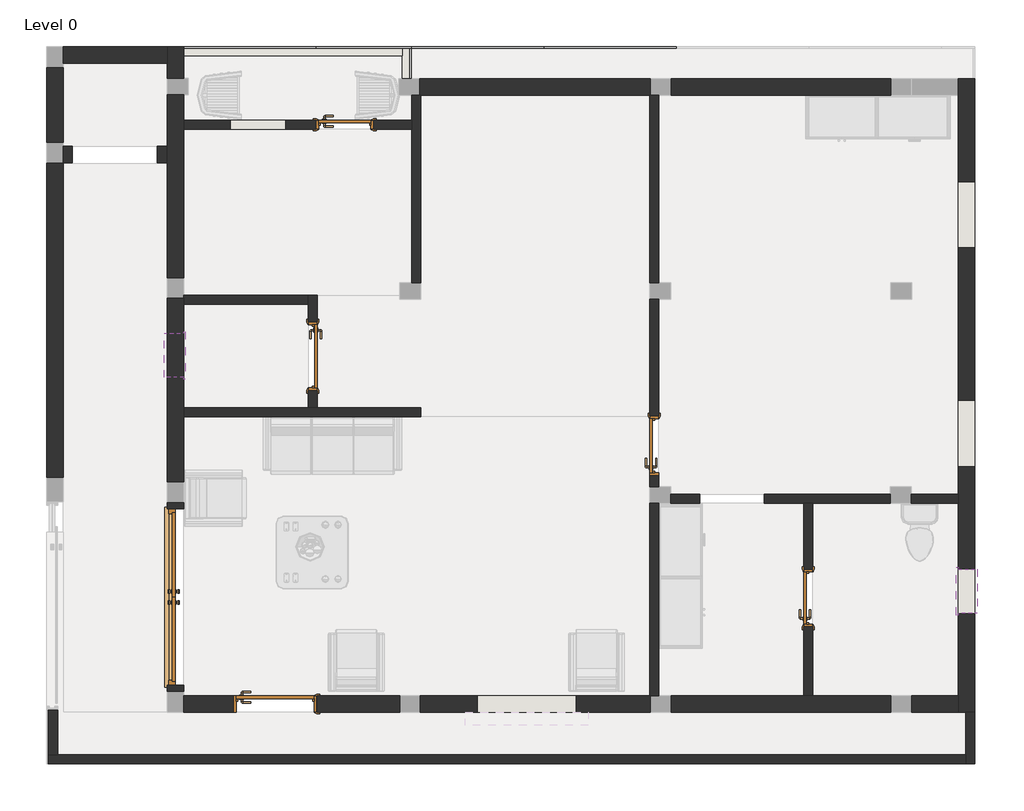
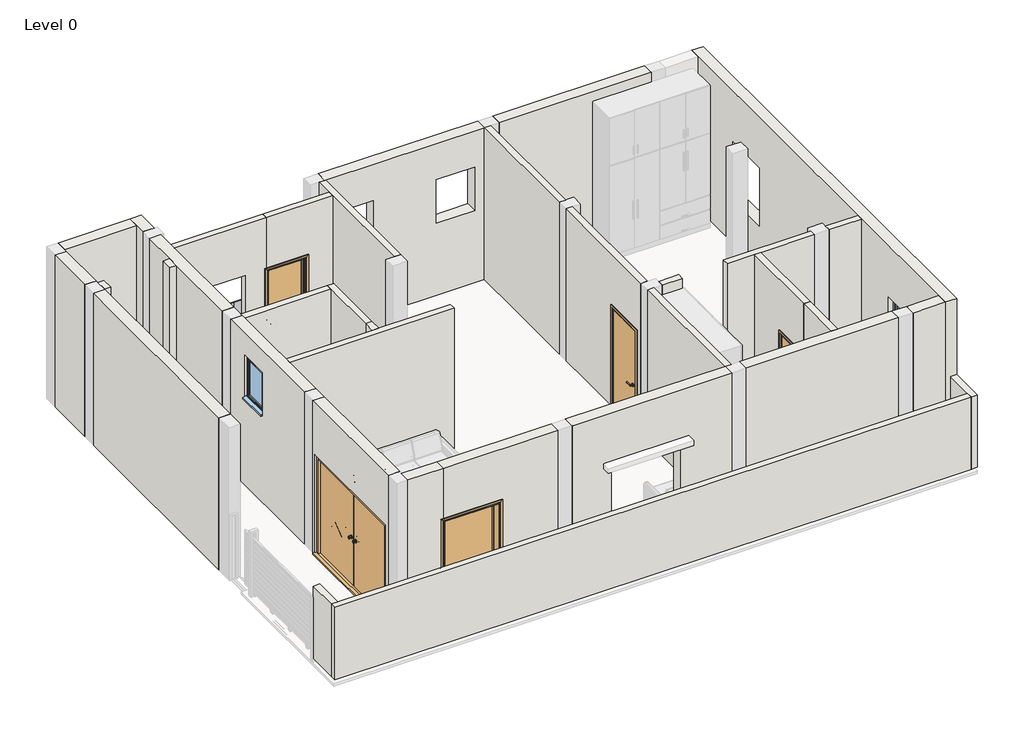
# One storey, part 1 of 2: 37 walls, 6 doors, 5 plates, 2 windows.
"""IFC4 building model written with IfcOpenShell, lengths in millimetres."""

from ifc_helpers import new_model, si_unit, frame, origin, origin_with_axes, place, context, project, spatial, polyline, outline, extrude, faceted_brep, transform, mapped, element, save
from components import doors_extdbl_flush_md_0ef74d11, doors_intsgl_d3_a25f8c6e, doors_intsgl_d4_4271d8f6, doors_intsgl_d1_afe1ebc3, doors_intsgl_d2_d6dd0e7a, system_panel_glazed_6338a664, system_panel_glazed_e6893c60, system_panel_glazed_bba74dcb, windows_sgl_plain_610x910mm_8d1346b0

model = new_model("IFC4")

# Units and contexts
model_context = context("Model", 3, world=origin())
ifc_project = project(units=[si_unit("LENGTHUNIT", "METRE", prefix="MILLI")], contexts=[model_context])

# Site, building, storey
site = spatial("IfcSite", under=ifc_project)
building = spatial("IfcBuilding", under=site)
storey = spatial("IfcBuildingStorey", under=building, Name="Level 0", Elevation=0.0)

# Doors
placement = place(None, origin())
doors_extdbl_flush_md_shape = doors_extdbl_flush_md_0ef74d11(model_context)
element("IfcDoor", 1, ObjectType="Doors_ExtDbl_Flush : MD", at=placement, inside=storey, context=model_context, shape_type="MappedRepresentation", body=[
    mapped(doors_extdbl_flush_md_shape, transform((-11061.4858712, -2060.9296054, 0.0), x_axis=(0.0, 1.0, 0.0), y_axis=(-1.0, 0.0, 0.0), z_axis=(0.0, 0.0, 1.0))),
])
doors_intsgl_d3_shape = doors_intsgl_d3_a25f8c6e(model_context)
element("IfcDoor", 2, ObjectType="Doors_IntSgl : D3", at=placement, inside=storey, context=model_context, shape_type="MappedRepresentation", body=[
    mapped(doors_intsgl_d3_shape, transform((-2315.0983223, -2074.5629976, 0.0), x_axis=(0.0, 1.0, 0.0), y_axis=(-1.0, 0.0, 0.0), z_axis=(0.0, 0.0, 1.0))),
])
element("IfcDoor", 3, ObjectType="Doors_IntSgl : D3", at=placement, inside=storey, context=model_context, shape_type="MappedRepresentation", body=[
    mapped(doors_intsgl_d3_shape, transform((-8718.3358712, 4467.3176487, 0.0), x_axis=(1.0, 0.0, 0.0), y_axis=(0.0, 1.0, 0.0), z_axis=(0.0, 0.0, 1.0))),
])
doors_intsgl_d4_shape = doors_intsgl_d4_4271d8f6(model_context)
element("IfcDoor", 4, ObjectType="Doors_IntSgl : D4", at=placement, inside=storey, context=model_context, shape_type="MappedRepresentation", body=[
    mapped(doors_intsgl_d4_shape, transform((-4442.6060272, 29.5702475, 0.0), x_axis=(0.0, 1.0, 0.0), y_axis=(-1.0, 0.0, 0.0), z_axis=(0.0, 0.0, 1.0))),
])
doors_intsgl_d1_shape = doors_intsgl_d1_afe1ebc3(model_context)
element("IfcDoor", 5, ObjectType="Doors_IntSgl : d1", at=placement, inside=storey, context=model_context, shape_type="MappedRepresentation", body=[
    mapped(doors_intsgl_d1_shape, transform((-9163.2845381, 1266.4703946, 0.0), x_axis=(0.0, -1.0, 0.0), y_axis=(1.0, 0.0, 0.0), z_axis=(0.0, 0.0, 1.0))),
])
doors_intsgl_d2_shape = doors_intsgl_d2_d6dd0e7a(model_context)
element("IfcDoor", 6, ObjectType="Doors_IntSgl : d2", at=placement, inside=storey, context=model_context, shape_type="MappedRepresentation", body=[
    mapped(doors_intsgl_d2_shape, transform((-9681.1945565, -3540.4796054, 0.0), x_axis=(1.0, 0.0, 0.0), y_axis=(0.0, 1.0, 0.0), z_axis=(0.0, 0.0, 1.0))),
])

# Plates
system_panel_glazed_shape = system_panel_glazed_6338a664(model_context)
element("IfcPlate", 7, ObjectType="System Panel : Glazed", at=placement, inside=storey, context=model_context, shape_type="MappedRepresentation", body=[
    mapped(system_panel_glazed_shape, transform((-10032.185871, 5496.5824405, 0.0), x_axis=(1.0, 0.0, 0.0), y_axis=(0.0, 1.0, 0.0), z_axis=(0.0, 0.0, 1.0))),
])
element("IfcPlate", 8, ObjectType="System Panel : Glazed", at=placement, inside=storey, context=model_context, shape_type="MappedRepresentation", body=[
    mapped(system_panel_glazed_shape, transform((-6883.885871, 5497.0125322, 0.0), x_axis=(1.0, 0.0, 0.0), y_axis=(0.0, 1.0, 0.0), z_axis=(0.0, 0.0, 1.0))),
])
element("IfcPlate", 9, ObjectType="System Panel : Glazed", at=placement, inside=storey, context=model_context, shape_type="MappedRepresentation", body=[
    mapped(system_panel_glazed_shape, transform((-5053.8858709, 5497.0125322, 0.0), x_axis=(1.0, 0.0, 0.0), y_axis=(0.0, 1.0, 0.0), z_axis=(0.0, 0.0, 1.0))),
])
system_panel_glazed_2_shape = system_panel_glazed_e6893c60(model_context)
element("IfcPlate", 10, ObjectType="System Panel : Glazed", at=placement, inside=storey, context=model_context, shape_type="MappedRepresentation", body=[
    mapped(system_panel_glazed_2_shape, transform((-8458.035871, 5496.5824405, 0.0), x_axis=(1.0, 0.0, 0.0), y_axis=(0.0, 1.0, 0.0), z_axis=(0.0, 0.0, 1.0))),
])
system_panel_glazed_3_shape = system_panel_glazed_bba74dcb(model_context)
element("IfcPlate", 11, ObjectType="System Panel : Glazed", at=placement, inside=storey, context=model_context, shape_type="MappedRepresentation", body=[
    mapped(system_panel_glazed_3_shape, transform((-7848.3858712, 5311.357594, 0.0), x_axis=(0.0, -1.0, 0.0), y_axis=(1.0, 0.0, 0.0), z_axis=(0.0, 0.0, 1.0))),
])

# Walls
element("IfcWall", 12, ObjectType="5\"", at=placement, inside=storey, context=model_context, shape_type="SweptSolid", body=[
    extrude(outline(polyline([(-10947.1858712, 5546.4824405), (-7926.5134981, 5546.4824405), (-7926.5134981, 5419.4824405), (-10947.1858712, 5419.4824405), (-10947.1858712, 5546.4824405)])), origin_with_axes(), (0.0, 0.0, 1.0), 76.2),
])
element("IfcWall", 13, ObjectType="5\"", at=placement, inside=storey, context=model_context, shape_type="SweptSolid", body=[
    extrude(outline(polyline([(-7926.5134981, 5101.6327475), (-7926.5134981, 5546.4824405), (-7799.5134981, 5546.4824405), (-7799.5134981, 5101.6327475), (-7926.5134981, 5101.6327475)])), origin_with_axes(), (0.0, 0.0, 1.0), 76.2),
])
element("IfcWall", 14, ObjectType="5\"", at=placement, inside=storey, context=model_context, shape_type="Brep", body=[
    faceted_brep([(-140.83523, -3654.7796054, 76.2), (-140.83523, -4238.9796054, 76.2), (-140.83523, -4365.9796054, 76.2), (-140.83523, -4365.9796054, 1600.2), (-140.83523, -4238.9796054, 1600.2), (-140.83523, -3654.7796054, 1600.2), (-13.83523, -3654.7796054, 76.2), (-13.83523, -3654.7796054, 1600.2), (-13.83523, -4365.9796054, 1600.2), (-13.83523, -4365.9796054, 76.2)], [[[0, 1, 2, 3, 4, 5]], [[6, 7, 8, 9]], [[2, 1, 0, 6, 9]], [[3, 2, 9, 8]], [[5, 4, 3, 8, 7]], [[0, 5, 7, 6]]]),
])
element("IfcWall", 15, ObjectType="5\"", at=placement, inside=storey, context=model_context, shape_type="Brep", body=[
    faceted_brep([(-140.83523, -4238.9796054, 76.2), (-12688.43523, -4238.9796054, 76.2), (-12815.43523, -4238.9796054, 76.2), (-12815.43523, -4238.9796054, 1600.2), (-12688.43523, -4238.9796054, 1600.2), (-140.83523, -4238.9796054, 1600.2), (-140.83523, -4365.9796054, 76.2), (-140.83523, -4365.9796054, 1600.2), (-12815.43523, -4365.9796054, 1600.2), (-12815.43523, -4365.9796054, 76.2)], [[[0, 1, 2, 3, 4, 5]], [[6, 7, 8, 9]], [[2, 1, 0, 6, 9]], [[3, 2, 9, 8]], [[5, 4, 3, 8, 7]], [[0, 5, 7, 6]]]),
])
element("IfcWall", 16, ObjectType="5\"", at=placement, inside=storey, context=model_context, shape_type="SweptSolid", body=[
    extrude(outline(polyline([(-12688.43523, -3623.9896501), (-12688.43523, -4238.9796054), (-12815.43523, -4238.9796054), (-12815.43523, -3623.9896501), (-12688.43523, -3623.9896501)])), frame((0.0, 0.0, 76.2), z_axis=(0.0, 0.0, 1.0), x_axis=(1.0, 0.0, 0.0)), (0.0, 0.0, 1.0), 1524.0),
])
element("IfcWall", 17, ObjectType="9\"", at=placement, inside=storey, context=model_context, shape_type="SweptSolid", body=[
    extrude(outline(polyline([(-12836.0604224, 4222.4988089), (-12836.0604224, 5253.6949405), (-12607.4604224, 5253.6949405), (-12607.4604224, 4222.4988089), (-12836.0604224, 4222.4988089)])), origin_with_axes(), (0.0, 0.0, 1.0), 3200.4),
])
element("IfcWall", 18, ObjectType="9\"", at=placement, inside=storey, context=model_context, shape_type="SweptSolid", body=[
    extrude(outline(polyline([(-12836.0604224, -404.5396501), (-12836.0604224, 3930.3988089), (-12607.4604224, 3930.3988089), (-12607.4604224, -404.5396501), (-12836.0604224, -404.5396501)])), origin_with_axes(), (0.0, 0.0, 1.0), 3200.4),
])
element("IfcWall", 19, ObjectType="9\"", at=placement, inside=storey, context=model_context, shape_type="SweptSolid", body=[
    extrude(outline(polyline([(3200.4, -10240.7910021), (3200.4, -10947.1858712), (0.0, -10947.1858712), (0.0, -10259.0445565), (2110.0, -10259.0445565), (2110.0, -10240.7910021), (3200.4, -10240.7910021)])), frame((0.0, -3654.7796054, 0.0), z_axis=(0.0, 1.0, 0.0), x_axis=(0.0, 0.0, 1.0)), (0.0, 0.0, 1.0), 228.6),
])
element("IfcWall", 20, ObjectType="9\"", at=placement, inside=storey, context=model_context, shape_type="SweptSolid", body=[
    extrude(outline(polyline([(0.0, -7960.3445565), (3200.4, -7960.3445565), (3200.4, -10240.7910021), (2110.0, -10240.7910021), (2110.0, -9103.3445565), (0.0, -9103.3445565), (0.0, -7960.3445565)])), frame((0.0, -3654.7796054, 0.0), z_axis=(0.0, 1.0, 0.0), x_axis=(0.0, 0.0, 1.0)), (0.0, 0.0, 1.0), 228.6),
])
element("IfcWall", 21, ObjectType="9\"", at=placement, inside=storey, context=model_context, shape_type="SweptSolid", body=[
    extrude(outline(polyline([(0.0, -7678.28523), (0.0, -4496.93523), (3200.4, -4496.93523), (3200.4, -7678.28523), (0.0, -7678.28523)]), holes=[polyline([(2133.6, -6890.88523), (2133.6, -5519.28523), (914.4, -5519.28523), (914.4, -6890.88523), (2133.6, -6890.88523)])]), frame((0.0, -3654.7796054, 0.0), z_axis=(0.0, 1.0, 0.0), x_axis=(0.0, 0.0, 1.0)), (0.0, 0.0, 1.0), 228.6),
])
element("IfcWall", 22, ObjectType="9\"", at=placement, inside=storey, context=model_context, shape_type="SweptSolid", body=[
    extrude(outline(polyline([(-1175.88523, -3654.7796054), (-4204.83523, -3654.7796054), (-4204.83523, -3426.1796054), (-1175.88523, -3426.1796054), (-1175.88523, -3654.7796054)])), origin_with_axes(), (0.0, 0.0, 1.0), 3200.4),
])
element("IfcWall", 23, ObjectType="9\"", at=placement, inside=storey, context=model_context, shape_type="SweptSolid", body=[
    extrude(outline(polyline([(-242.43523, -3654.7796054), (-883.78523, -3654.7796054), (-883.78523, -3426.1796054), (-242.43523, -3426.1796054), (-242.43523, -3654.7796054)])), origin_with_axes(), (0.0, 0.0, 1.0), 3200.4),
])
element("IfcWall", 24, ObjectType="9\"", at=placement, inside=storey, context=model_context, shape_type="Brep", body=[
    faceted_brep([(-13.83523, -3654.7796054, 0.0), (-13.83523, 5101.6327475, 0.0), (-13.83523, 5101.6327475, 3200.4), (-13.83523, -3654.7796054, 3200.4), (-13.83523, -3654.7796054, 1600.2), (-13.83523, -3654.7796054, 76.2), (-13.83523, 2764.8327475, 2133.6), (-13.83523, 3679.2327475, 2133.6), (-13.83523, 3679.2327475, 914.4), (-13.83523, 2764.8327475, 914.4), (-13.83523, -257.7672525, 2133.6), (-13.83523, 656.6327475, 2133.6), (-13.83523, 656.6327475, 914.4), (-13.83523, -257.7672525, 914.4), (-13.83523, -1676.8734289, 2110.0), (-13.83523, -1676.8734289, 1200.0), (-13.83523, -2286.4734289, 1200.0), (-13.83523, -2286.4734289, 2110.0), (-242.43523, -3654.7796054, 0.0), (-242.43523, -3654.7796054, 3200.4), (-242.43523, -3426.1796054, 3200.4), (-242.43523, 4873.0327475, 3200.4), (-242.43523, 5101.6327475, 3200.4), (-242.43523, 5101.6327475, 0.0), (-242.43523, 4873.0327475, 0.0), (-242.43523, -3426.1796054, 0.0), (-242.43523, 2764.8327475, 2133.6), (-242.43523, 2764.8327475, 914.4), (-242.43523, 3679.2327475, 914.4), (-242.43523, 3679.2327475, 2133.6), (-242.43523, -257.7672525, 2133.6), (-242.43523, -257.7672525, 914.4), (-242.43523, 656.6327475, 914.4), (-242.43523, 656.6327475, 2133.6), (-242.43523, -1676.8734289, 2110.0), (-242.43523, -2286.4734289, 2110.0), (-242.43523, -2286.4734289, 1200.0), (-242.43523, -1676.8734289, 1200.0)], [[[0, 1, 2, 3, 4, 5], [6, 7, 8, 9], [10, 11, 12, 13], [14, 15, 16, 17]], [[18, 19, 20, 21, 22, 23, 24, 25], [26, 27, 28, 29], [30, 31, 32, 33], [34, 35, 36, 37]], [[1, 0, 18, 25, 24, 23]], [[2, 1, 23, 22]], [[3, 2, 22, 21, 20, 19]], [[0, 5, 4, 3, 19, 18]], [[27, 26, 6, 9]], [[28, 27, 9, 8]], [[29, 28, 8, 7]], [[26, 29, 7, 6]], [[31, 30, 10, 13]], [[32, 31, 13, 12]], [[33, 32, 12, 11]], [[30, 33, 11, 10]], [[15, 14, 34, 37]], [[16, 15, 37, 36]], [[17, 16, 36, 35]], [[14, 17, 35, 34]]]),
])
element("IfcWall", 25, ObjectType="9\"", at=placement, inside=storey, context=model_context, shape_type="SweptSolid", body=[
    extrude(outline(polyline([(-4207.375513, 5101.6327475), (-1175.88523, 5101.6327475), (-1175.88523, 4873.0327475), (-4207.375513, 4873.0327475), (-4207.375513, 5101.6327475)])), origin_with_axes(), (0.0, 0.0, 1.0), 3200.4),
])
element("IfcWall", 26, ObjectType="9\"", at=placement, inside=storey, context=model_context, shape_type="Brep", body=[
    faceted_brep([(-4499.475513, 5101.6327475, 0.0), (-7680.825513, 5101.6327475, 0.0), (-7680.825513, 5101.6327475, 3200.4), (-4499.475513, 5101.6327475, 3200.4), (-7477.625513, 5101.6327475, 2438.4), (-7477.625513, 5101.6327475, 1524.0), (-6715.625513, 5101.6327475, 1524.0), (-6715.625513, 5101.6327475, 2438.4), (-5458.325513, 5101.6327475, 2438.4), (-5458.325513, 5101.6327475, 1524.0), (-4696.325513, 5101.6327475, 1524.0), (-4696.325513, 5101.6327475, 2438.4), (-4499.475513, 4873.0327475, 0.0), (-4499.475513, 4873.0327475, 3200.4), (-7666.1634981, 4873.0327475, 3200.4), (-7680.825513, 4873.0327475, 3200.4), (-7680.825513, 4873.0327475, 0.0), (-7666.1634981, 4873.0327475, 0.0), (-7477.625513, 4873.0327475, 2438.4), (-6715.625513, 4873.0327475, 2438.4), (-6715.625513, 4873.0327475, 1524.0), (-7477.625513, 4873.0327475, 1524.0), (-5458.325513, 4873.0327475, 2438.4), (-4696.325513, 4873.0327475, 2438.4), (-4696.325513, 4873.0327475, 1524.0), (-5458.325513, 4873.0327475, 1524.0)], [[[0, 1, 2, 3], [4, 5, 6, 7], [8, 9, 10, 11]], [[12, 13, 14, 15, 16, 17], [18, 19, 20, 21], [22, 23, 24, 25]], [[1, 0, 12, 17, 16]], [[2, 1, 16, 15]], [[3, 2, 15, 14, 13]], [[0, 3, 13, 12]], [[5, 4, 18, 21]], [[6, 5, 21, 20]], [[7, 6, 20, 19]], [[4, 7, 19, 18]], [[9, 8, 22, 25]], [[10, 9, 25, 24]], [[11, 10, 24, 23]], [[8, 11, 23, 22]]]),
])
element("IfcWall", 27, ObjectType="9\"", at=placement, inside=storey, context=model_context, shape_type="SweptSolid", body=[
    extrude(outline(polyline([(-11175.7858712, 5317.1949405), (-12607.4604224, 5317.1949405), (-12607.4604224, 5545.7949405), (-11175.7858712, 5545.7949405), (-11175.7858712, 5317.1949405)])), origin_with_axes(), (0.0, 0.0, 1.0), 3200.4),
])
element("IfcWall", 28, ObjectType="9\"", at=placement, inside=storey, context=model_context, shape_type="Brep", body=[
    faceted_brep([(-11175.7858712, 5545.7949405, 0.0), (-11175.7858712, 5317.1949405, 0.0), (-11175.7858712, 5105.4926487, 0.0), (-11175.7858712, 5105.4926487, 3200.4), (-11175.7858712, 5317.1949405, 3200.4), (-11175.7858712, 5545.7949405, 3200.4), (-10947.1858712, 5545.7949405, 0.0), (-10947.1858712, 5545.7949405, 3200.4), (-10947.1858712, 5105.4926487, 3200.4), (-10947.1858712, 5105.4926487, 0.0)], [[[0, 1, 2, 3, 4, 5]], [[6, 7, 8, 9]], [[2, 1, 0, 6, 9]], [[3, 2, 9, 8]], [[5, 4, 3, 8, 7]], [[0, 5, 7, 6]]]),
])
element("IfcWall", 29, ObjectType="9\"", at=placement, inside=storey, context=model_context, shape_type="Brep", body=[
    faceted_brep([(-11175.7858712, 4876.8926487, 0.0), (-11175.7858712, 4168.5238089, 0.0), (-11175.7858712, 3939.9238089, 0.0), (-11175.7858712, 2353.0673305, 0.0), (-11175.7858712, 2353.0673305, 3200.4), (-11175.7858712, 3939.9238089, 3200.4), (-11175.7858712, 4168.5238089, 3200.4), (-11175.7858712, 4876.8926487, 3200.4), (-10947.1858712, 4876.8926487, 0.0), (-10947.1858712, 4876.8926487, 3200.4), (-10947.1858712, 4530.8176487, 3200.4), (-10947.1858712, 4403.8176487, 3200.4), (-10947.1858712, 2353.0673305, 3200.4), (-10947.1858712, 2353.0673305, 0.0), (-10947.1858712, 4403.8176487, 0.0), (-10947.1858712, 4530.8176487, 0.0)], [[[0, 1, 2, 3, 4, 5, 6, 7]], [[8, 9, 10, 11, 12, 13, 14, 15]], [[3, 2, 1, 0, 8, 15, 14, 13]], [[4, 3, 13, 12]], [[7, 6, 5, 4, 12, 11, 10, 9]], [[0, 7, 9, 8]]]),
])
element("IfcWall", 30, ObjectType="9\"", at=placement, inside=storey, context=model_context, shape_type="SweptSolid", body=[
    extrude(outline(polyline([(2065.5455124, 0.0), (-467.0796054, 0.0), (-467.0796054, 3200.4), (2065.5455124, 3200.4), (2065.5455124, 0.0)]), holes=[polyline([(973.3455124, 2738.8), (973.3455124, 1828.8), (1582.9455124, 1828.8), (1582.9455124, 2738.8), (973.3455124, 2738.8)])]), frame((-11175.7858712, 0.0, 0.0), z_axis=(1.0, 0.0, 0.0), x_axis=(0.0, 1.0, 0.0)), (0.0, 0.0, 1.0), 228.6),
])
element("IfcWall", 31, ObjectType="9\"", at=placement, inside=storey, context=model_context, shape_type="SweptSolid", body=[
    extrude(outline(polyline([(-759.1796054, 0.0), (-841.7296054, 0.0), (-841.7296054, 2110.0), (-3280.1296054, 2110.0), (-3280.1296054, 0.0), (-3362.6796054, 0.0), (-3362.6796054, 3200.4), (-759.1796054, 3200.4), (-759.1796054, 0.0)])), frame((-11175.7858712, 0.0, 0.0), z_axis=(1.0, 0.0, 0.0), x_axis=(0.0, 1.0, 0.0)), (0.0, 0.0, 1.0), 228.6),
])
element("IfcWall", 32, ObjectType="9\"", at=placement, inside=storey, context=model_context, shape_type="SweptSolid", body=[
    extrude(outline(polyline([(-12486.8104224, 3939.9238089), (-12607.4604224, 3939.9238089), (-12607.4604224, 4168.5238089), (-12486.8104224, 4168.5238089), (-12486.8104224, 3939.9238089)])), origin_with_axes(), (0.0, 0.0, 1.0), 3200.4),
])
element("IfcWall", 33, ObjectType="9\"", at=placement, inside=storey, context=model_context, shape_type="SweptSolid", body=[
    extrude(outline(polyline([(-11175.7858712, 3939.9238089), (-11308.4687707, 3939.9238089), (-11308.4687707, 4168.5238089), (-11175.7858712, 4168.5238089), (-11175.7858712, 3939.9238089)])), origin_with_axes(), (0.0, 0.0, 1.0), 3200.4),
])
element("IfcWall", 34, ObjectType="brick 5\"", at=placement, inside=storey, context=model_context, shape_type="SweptSolid", body=[
    extrude(outline(polyline([(0.0, -10947.1858712), (0.0, -9118.3858712), (3200.4, -9118.3858712), (3200.4, -10947.1858712), (0.0, -10947.1858712)]), holes=[polyline([(2133.6, -10299.4858712), (2133.6, -9537.4858712), (914.4, -9537.4858712), (914.4, -10299.4858712), (2133.6, -10299.4858712)])]), frame((0.0, 4403.8176487, 0.0), z_axis=(0.0, 1.0, 0.0), x_axis=(0.0, 0.0, 1.0)), (0.0, 0.0, 1.0), 127.0),
])
element("IfcWall", 35, ObjectType="brick 5\"", at=placement, inside=storey, context=model_context, shape_type="SweptSolid", body=[
    extrude(outline(polyline([(0.0, -7793.1634981), (3200.4, -7793.1634981), (3200.4, -9118.3858712), (2110.0, -9118.3858712), (2110.0, -8318.2858712), (0.0, -8318.2858712), (0.0, -7793.1634981)])), frame((0.0, 4403.8176487, 0.0), z_axis=(0.0, 1.0, 0.0), x_axis=(0.0, 0.0, 1.0)), (0.0, 0.0, 1.0), 127.0),
])
element("IfcWall", 36, ObjectType="brick 5\"", at=placement, inside=storey, context=model_context, shape_type="Brep", body=[
    faceted_brep([(-7793.1634981, 4873.0327475, 0.0), (-7793.1634981, 4530.8176487, 0.0), (-7793.1634981, 4403.8176487, 0.0), (-7793.1634981, 2285.4077475, 0.0), (-7793.1634981, 2285.4077475, 3200.4), (-7793.1634981, 4403.8176487, 3200.4), (-7793.1634981, 4530.8176487, 3200.4), (-7793.1634981, 4873.0327475, 3200.4), (-7666.1634981, 4873.0327475, 0.0), (-7666.1634981, 4873.0327475, 3200.4), (-7666.1634981, 2285.4077475, 3200.4), (-7666.1634981, 2285.4077475, 0.0), (-7680.825513, 4873.0327475, 0.0), (-7680.825513, 4873.0327475, 3200.4)], [[[0, 1, 2, 3, 4, 5, 6, 7]], [[8, 9, 10, 11]], [[3, 2, 1, 0, 12, 8, 11]], [[4, 3, 11, 10]], [[7, 6, 5, 4, 10, 9, 13]], [[0, 7, 13, 9, 8, 12]]]),
])
element("IfcWall", 37, ObjectType="brick 5\"", at=placement, inside=storey, context=model_context, shape_type="SweptSolid", body=[
    extrude(outline(polyline([(-9226.7845381, 1983.7280605), (-10947.1858712, 1983.7280605), (-10947.1858712, 2110.7280605), (-9226.7845381, 2110.7280605), (-9226.7845381, 1983.7280605)])), origin_with_axes(), (0.0, 0.0, 1.0), 3200.4),
])
element("IfcWall", 38, ObjectType="brick 5\"", at=placement, inside=storey, context=model_context, shape_type="Brep", body=[
    faceted_brep([(-9226.7845381, 790.2203946, 3200.4), (-9226.7845381, 1983.7280605, 3200.4), (-9226.7845381, 2110.7280605, 3200.4), (-9226.7845381, 2110.7280605, 0.0), (-9226.7845381, 1983.7280605, 0.0), (-9226.7845381, 1742.7203946, 0.0), (-9226.7845381, 1742.7203946, 2110.0), (-9226.7845381, 790.2203946, 2110.0), (-9099.7845381, 2110.7280605, 3200.4), (-9099.7845381, 790.2203946, 3200.4), (-9099.7845381, 790.2203946, 2110.0), (-9099.7845381, 1742.7203946, 2110.0), (-9099.7845381, 1742.7203946, 0.0), (-9099.7845381, 2110.7280605, 0.0)], [[[0, 1, 2, 3, 4, 5, 6, 7]], [[8, 9, 10, 11, 12, 13]], [[3, 13, 12, 5, 4]], [[9, 0, 7, 10]], [[2, 1, 0, 9, 8]], [[3, 2, 8, 13]], [[6, 11, 10, 7]], [[11, 6, 5, 12]]]),
])
element("IfcWall", 39, ObjectType="brick 5\"", at=placement, inside=storey, context=model_context, shape_type="Brep", body=[
    faceted_brep([(-10947.1858712, 428.2703946, 0.0), (-7670.5858712, 428.2703946, 0.0), (-7670.5858712, 428.2703946, 3200.4), (-10947.1858712, 428.2703946, 3200.4), (-10947.1858712, 555.2703946, 0.0), (-10947.1858712, 555.2703946, 3200.4), (-9226.3358712, 555.2703946, 3200.4), (-9099.3358712, 555.2703946, 3200.4), (-7670.5858712, 555.2703946, 3200.4), (-7670.5858712, 555.2703946, 0.0), (-9099.3358712, 555.2703946, 0.0), (-9226.3358712, 555.2703946, 0.0)], [[[0, 1, 2, 3]], [[4, 5, 6, 7, 8, 9, 10, 11]], [[1, 0, 4, 11, 10, 9]], [[2, 1, 9, 8]], [[3, 2, 8, 7, 6, 5]], [[0, 3, 5, 4]]]),
])
element("IfcWall", 40, ObjectType="brick 5\"", at=placement, inside=storey, context=model_context, shape_type="SweptSolid", body=[
    extrude(outline(polyline([(-9099.3358712, 790.2203946), (-9099.3358712, 555.2703946), (-9226.3358712, 555.2703946), (-9226.3358712, 790.2203946), (-9099.3358712, 790.2203946)])), origin_with_axes(), (0.0, 0.0, 1.0), 3200.4),
])
element("IfcWall", 41, ObjectType="brick 5\"", at=placement, inside=storey, context=model_context, shape_type="SweptSolid", body=[
    extrude(outline(polyline([(-4506.1060272, 2285.4077475), (-4506.1060272, 4873.0327475), (-4379.1060272, 4873.0327475), (-4379.1060272, 2285.4077475), (-4506.1060272, 2285.4077475)])), origin_with_axes(), (0.0, 0.0, 1.0), 3200.4),
])
element("IfcWall", 42, ObjectType="brick 5\"", at=placement, inside=storey, context=model_context, shape_type="SweptSolid", body=[
    extrude(outline(polyline([(-535.5797525, 0.0), (-535.5797525, 3200.4), (2056.8077475, 3200.4), (2056.8077475, 0.0), (442.3202475, 0.0), (442.3202475, 2110.0), (-383.1797525, 2110.0), (-383.1797525, 0.0), (-535.5797525, 0.0)])), frame((-4506.1060272, 0.0, 0.0), z_axis=(1.0, 0.0, 0.0), x_axis=(0.0, 1.0, 0.0)), (0.0, 0.0, 1.0), 127.0),
])
element("IfcWall", 43, ObjectType="brick 5\"", at=placement, inside=storey, context=model_context, shape_type="SweptSolid", body=[
    extrude(outline(polyline([(-4506.1060272, -3426.1796054), (-4506.1060272, -764.1797525), (-4379.1060272, -764.1797525), (-4379.1060272, -3426.1796054), (-4506.1060272, -3426.1796054)])), origin_with_axes(), (0.0, 0.0, 1.0), 3200.4),
])
element("IfcWall", 44, ObjectType="brick 5\"", at=placement, inside=storey, context=model_context, shape_type="SweptSolid", body=[
    extrude(outline(polyline([(-3813.9560272, -764.1797525), (-4214.0060272, -764.1797525), (-4214.0060272, -637.1797525), (-3813.9560272, -637.1797525), (-3813.9560272, -764.1797525)])), origin_with_axes(), (0.0, 0.0, 1.0), 3200.4),
])
element("IfcWall", 45, ObjectType="brick 5\"", at=placement, inside=storey, context=model_context, shape_type="Brep", body=[
    faceted_brep([(-2920.6153893, -764.1797525, 0.0), (-2378.5983223, -764.1797525, 0.0), (-2251.5983223, -764.1797525, 0.0), (-1182.23523, -764.1797525, 0.0), (-1182.23523, -764.1797525, 3200.4), (-2251.5983223, -764.1797525, 3200.4), (-2378.5983223, -764.1797525, 3200.4), (-2920.6153893, -764.1797525, 3200.4), (-2920.6153893, -637.1797525, 0.0), (-2920.6153893, -637.1797525, 3200.4), (-1182.23523, -637.1797525, 3200.4), (-1182.23523, -637.1797525, 0.0)], [[[0, 1, 2, 3, 4, 5, 6, 7]], [[8, 9, 10, 11]], [[3, 2, 1, 0, 8, 11]], [[4, 3, 11, 10]], [[7, 6, 5, 4, 10, 9]], [[0, 7, 9, 8]]]),
])
element("IfcWall", 46, ObjectType="brick 5\"", at=placement, inside=storey, context=model_context, shape_type="SweptSolid", body=[
    extrude(outline(polyline([(-242.43523, -764.1797525), (-890.13523, -764.1797525), (-890.13523, -637.1797525), (-242.43523, -637.1797525), (-242.43523, -764.1797525)])), origin_with_axes(), (0.0, 0.0, 1.0), 3200.4),
])
element("IfcWall", 47, ObjectType="brick 5\"", at=placement, inside=storey, context=model_context, shape_type="SweptSolid", body=[
    extrude(outline(polyline([(-2474.6129976, 3200.4), (-764.1797525, 3200.4), (-764.1797525, 0.0), (-1674.5129976, 0.0), (-1674.5129976, 2110.0), (-2474.6129976, 2110.0), (-2474.6129976, 3200.4)])), frame((-2378.5983223, 0.0, 0.0), z_axis=(1.0, 0.0, 0.0), x_axis=(0.0, 1.0, 0.0)), (0.0, 0.0, 1.0), 127.0),
])
element("IfcWall", 48, ObjectType="brick 5\"", at=placement, inside=storey, context=model_context, shape_type="SweptSolid", body=[
    extrude(outline(polyline([(-2378.5983223, -3426.1796054), (-2378.5983223, -2474.6129976), (-2251.5983223, -2474.6129976), (-2251.5983223, -3426.1796054), (-2378.5983223, -3426.1796054)])), origin_with_axes(), (0.0, 0.0, 1.0), 3200.4),
])

# Windows
windows_sgl_plain_610x910mm_shape = windows_sgl_plain_610x910mm_8d1346b0(model_context)
element("IfcWindow", 49, ObjectType="Windows_Sgl_Plain : 610x910mm", at=placement, inside=storey, context=model_context, shape_type="MappedRepresentation", body=[
    mapped(windows_sgl_plain_610x910mm_shape, transform((-11053.0293033, 1278.1455124, 628.8), x_axis=(0.0, 1.0, 0.0), y_axis=(-1.0, 0.0, 0.0), z_axis=(0.0, 0.0, 1.0))),
])
element("IfcWindow", 50, ObjectType="Windows_Sgl_Plain : 610x910mm", at=placement, inside=storey, context=model_context, shape_type="MappedRepresentation", body=[
    mapped(windows_sgl_plain_610x910mm_shape, transform((-136.5917978, -1981.6734289, 0.0), x_axis=(0.0, -1.0, 0.0), y_axis=(1.0, 0.0, 0.0), z_axis=(0.0, 0.0, 1.0))),
])

save(model, "model.ifc")

# Revit data of these elements
# Type "Doors_ExtDbl_Flush : MD"
#   Type Mark = "47"
#   Type Comments = "External Double"
#   Operation = "DoubleDoorSingleSwing"
#   Keynote = "L20"
#   Analytic Construction = "Metal"
#   Wrap Layers (Ext) from Ext = 0' - 4.03543"
#   Wrap Layers (Int) from Ext = 0' - 6.98819"
#   Thickness = 0' - 1.73228"
#   Rough Width = 8' - 0"
#   Rough Height = 6' - 11.07087"
#   O/A Frame Width = 0' - 2.51969"
#   Heat Transfer Coefficient (U) = 3.7021 W/(m²·K)
#   Handle Z Distance = 3' - 5.33858"
#   FrameWidth = 0' - 1.65354"
#   FrameOffset - External = 0' - 0.98425"
#   FrameDepth = 0' - 3.50394"
#   Door Panel Width = 3' - 9.91339"
#   Door Panel Thickness = 0' - 1.73228"
#   Door Panel Height = 6' - 6.74016"
#   Cill Thickness = 0' - 2.14567"
#   Cill Projection = 0' - 1.1811"
#   Handle X Distance = 0' - 2.95276"
#   Height = 6' - 11.07087"
#   Structural Tolerance = 0' - 0.25591"
#   Tolerance = 0' - 0.11811"
#   Undercut = 0' - 0.15748"
#   Width = 8' - 0"
#   Cill Extension = 0' - 0.98425"
#   Cavity Closer Width = 0' - 1.9685"
#   Cavity Closer Offset from Ext = 0' - 4.03543"
#   Cavity Closer Depth = 0' - 3.34646"
#   Vis - Ironmongery = yes
#   Vis - Cavity Closers = yes
#   Function = 1
#   Material Door = Door - Panel
#   Material Frame = Door - Frame/Mullion
#   Material Ironmongery = Door - Handle
#   Visual Light Transmittance = 0
#   Thermal Resistance (R) = 0
#   Solar Heat Gain Coefficient = 0
#   Wall Closure = (empty or 0)
# Type "Doors_IntSgl : D3"
#   Type Mark = "49"
#   Type Comments = "Internal Single"
#   Operation = "SingleSwingRight"
#   Manufacturer = "Revit"
#   Keynote = "L20"
#   Description = "Internal Single Door"
#   Analytic Construction = "Metal"
#   UnderCut = 0' - 0.31496"
#   Tolerance = 0' - 0.07874"
#   Thickness = 0' - 1.49606"
#   Thermal Resistance (R) = 0.270117 (m²·K)/W
#   Structural Tolerance = 0' - 0.31496"
#   StopDepth = 0' - 1.25984"
#   Stop Thickness = 0' - 0.74803"
#   Rough Width = 2' - 7 1/2"
#   Rough Height = 6' - 11.07087"
#   Height to Top Lock Rail = 3' - 3.37008"
#   Heat Transfer Coefficient (U) = 3.7021 W/(m²·K)
#   Handle Z Distance = 2' - 11.43307"
#   Handle X Distance = 0' - 2.95276"
#   Frame Thickness = 0' - 1.25984"
#   Door Panel Width = 2' - 4.19291"
#   Door Panel Thickness = 0' - 1.49606"
#   Door Panel Offset = 0' - 0"
#   Height = 6' - 11.07087"
#   Width = 2' - 7 1/2"
#   Door Panel Height = 6' - 9.10236"
#   Architrave Setback = 0' - 0.19685"
#   Vis - Ironmongery = yes
#   Material Ironmongery = Door - Handle
#   Material Frame = Door - Frame/Mullion (1)
#   Material Door = Door - Panel
#   Material Architrave = Door - Architrave
#   Visual Light Transmittance = 0
#   Solar Heat Gain Coefficient = 0
#   Function = (empty or 0)
#   Wall Closure = (empty or 0)
# Type "Doors_IntSgl : D4"
#   Type Mark = "50"
#   Type Comments = "Internal Single"
#   Operation = "SingleSwingRight"
#   Manufacturer = "Revit"
#   Keynote = "L20"
#   Description = "Internal Single Door"
#   Analytic Construction = "Metal"
#   UnderCut = 0' - 0.31496"
#   Tolerance = 0' - 0.07874"
#   Thickness = 0' - 1.49606"
#   Thermal Resistance (R) = 0.270117 (m²·K)/W
#   Structural Tolerance = 0' - 0.31496"
#   StopDepth = 0' - 1.25984"
#   Stop Thickness = 0' - 0.74803"
#   Rough Width = 2' - 8 1/2"
#   Rough Height = 6' - 11.07087"
#   Height to Top Lock Rail = 3' - 3.37008"
#   Heat Transfer Coefficient (U) = 3.7021 W/(m²·K)
#   Handle Z Distance = 2' - 11.43307"
#   Handle X Distance = 0' - 2.95276"
#   Frame Thickness = 0' - 1.25984"
#   Door Panel Width = 2' - 5.19291"
#   Door Panel Thickness = 0' - 1.49606"
#   Door Panel Offset = 0' - 0"
#   Height = 6' - 11.07087"
#   Width = 2' - 8 1/2"
#   Door Panel Height = 6' - 9.10236"
#   Architrave Setback = 0' - 0.19685"
#   Vis - Ironmongery = yes
#   Material Ironmongery = Door - Handle
#   Material Frame = Door - Frame/Mullion (1)
#   Material Door = Door - Panel
#   Material Architrave = Door - Architrave
#   Visual Light Transmittance = 0
#   Solar Heat Gain Coefficient = 0
#   Function = (empty or 0)
#   Wall Closure = (empty or 0)
# Type "Doors_IntSgl : d1"
#   Type Mark = "46"
#   Type Comments = "Internal Single"
#   Operation = "SingleSwingRight"
#   Manufacturer = "Revit"
#   Keynote = "L20"
#   Description = "Internal Single Door"
#   Analytic Construction = "Metal"
#   UnderCut = 0' - 0.31496"
#   Tolerance = 0' - 0.07874"
#   Thickness = 0' - 1.49606"
#   Thermal Resistance (R) = 0.270117 (m²·K)/W
#   Structural Tolerance = 0' - 0.31496"
#   StopDepth = 0' - 1.25984"
#   Stop Thickness = 0' - 0.74803"
#   Rough Width = 3' - 1 1/2"
#   Rough Height = 6' - 11.07087"
#   Height to Top Lock Rail = 3' - 3.37008"
#   Heat Transfer Coefficient (U) = 3.7021 W/(m²·K)
#   Handle Z Distance = 2' - 11.43307"
#   Handle X Distance = 0' - 2.95276"
#   Frame Thickness = 0' - 1.25984"
#   Door Panel Width = 2' - 10.19291"
#   Door Panel Thickness = 0' - 1.49606"
#   Door Panel Offset = 0' - 0"
#   Height = 6' - 11.07087"
#   Width = 3' - 1 1/2"
#   Door Panel Height = 6' - 9.10236"
#   Architrave Setback = 0' - 0.19685"
#   Vis - Ironmongery = yes
#   Material Ironmongery = Door - Handle
#   Material Frame = Door - Frame/Mullion (1)
#   Material Door = Door - Panel
#   Material Architrave = Door - Architrave
#   Visual Light Transmittance = 0
#   Solar Heat Gain Coefficient = 0
#   Function = (empty or 0)
#   Wall Closure = (empty or 0)
# Type "Doors_IntSgl : d2"
#   Type Mark = "48"
#   Type Comments = "Internal Single"
#   Operation = "SingleSwingRight"
#   Manufacturer = "Revit"
#   Keynote = "L20"
#   Description = "Internal Single Door"
#   Analytic Construction = "Metal"
#   UnderCut = 0' - 0.31496"
#   Tolerance = 0' - 0.07874"
#   Thickness = 0' - 1.49606"
#   Thermal Resistance (R) = 0.270117 (m²·K)/W
#   Structural Tolerance = 0' - 0.31496"
#   StopDepth = 0' - 1.25984"
#   Stop Thickness = 0' - 0.74803"
#   Rough Width = 3' - 9 1/2"
#   Rough Height = 6' - 11.07087"
#   Height to Top Lock Rail = 3' - 3.37008"
#   Heat Transfer Coefficient (U) = 3.7021 W/(m²·K)
#   Handle Z Distance = 2' - 11.43307"
#   Handle X Distance = 0' - 2.95276"
#   Frame Thickness = 0' - 1.25984"
#   Door Panel Width = 3' - 6.19291"
#   Door Panel Thickness = 0' - 1.49606"
#   Door Panel Offset = 0' - 0"
#   Height = 6' - 11.07087"
#   Width = 3' - 9 1/2"
#   Door Panel Height = 6' - 9.10236"
#   Architrave Setback = 0' - 0.19685"
#   Vis - Ironmongery = yes
#   Material Ironmongery = Door - Handle
#   Material Frame = Door - Frame/Mullion (1)
#   Material Door = Door - Panel
#   Material Architrave = Door - Architrave
#   Visual Light Transmittance = 0
#   Solar Heat Gain Coefficient = 0
#   Function = (empty or 0)
#   Wall Closure = (empty or 0)
# Type "System Panel : Glazed"
#   Keynote = "H11"
#   Construction Type Id = "GSP4R"
#   Analytic Construction = "1/8 in Pilkington single glazing"
#   Visual Light Transmittance = 0.9
#   Solar Heat Gain Coefficient = 0.86
#   Heat Transfer Coefficient (U) = 6.7069 W/(m²·K)
#   Define Thermal Properties by = 1
# Type "5\""
#   Keynote = "F10"
#   Layers, outside or top first: 0' - 5" "Concrete" (function 1)
# Type "9\""
#   Keynote = "F10"
#   Layers, outside or top first: 0' - 9" "Concrete" (function 1)
# Type "brick 5\""
#   Keynote = "F10"
#   Layers, outside or top first: 0' - 5" "Brick, Engineering" (function 1)
# Type "Windows_Sgl_Plain : 610x910mm"
#   Type Mark = "44"
#   Operation = "SinglePanel"
#   Construction Type Id = "SGL"
#   Manufacturer = "Revit"
#   Keynote = "L10"
#   Analytic Construction = "Large single-glazed windows"
#   Wrap Layers (Ext) from Ext = 0' - 4.03543"
#   Wrap Layers (Int) from Ext = 0' - 6.98819"
#   Window Board Projection = 0' - 0.98425"
#   Window Board Extension = 0' - 0.98425"
#   Visual Light Transmittance = 0.9
#   Solar Heat Gain Coefficient = 0.86
#   Rough Width = 2' - 0"
#   Rough Height = 2' - 11.82677"
#   Height = 2' - 11.82677"
#   Width = 2' - 0"
#   Heat Transfer Coefficient (U) = 5.5617 W/(m²·K)
#   Glazing Thickness = 0' - 0.94488"
#   FrameOffset - External = 0' - 1.9685"
#   Frame Depth = 0' - 2.55906"
#   Default Head Height = 6' - 11.07087"
#   Cill Depth = 0' - 3.44488"
#   Cavity Closer Width = 0' - 1.9685"
#   Cavity Closer Offset from Ext = 0' - 4.03543"
#   Cavity Closer Depth = 0' - 3.34646"
#   Define Thermal Properties by = 1
#   Vis - Cavity Closers = yes
#   Define Thermal Properties by = 1
#   Material Trim = Window Frame
#   Material Glass = Glass
#   Material Frame = Window Frame
#   Wall Closure = (empty or 0)
# Element 1 (IfcDoor, "Doors_ExtDbl_Flush : MD")
#   Phase Created = New Construction
#   Materials on its faces: "Door - Handle", "Door - Frame/Mullion", "Door - Panel"
# Elements 2, 3 (IfcDoor, "Doors_IntSgl : D3")
#   Phase Created = New Construction
#   Materials on its faces: "Door - Architrave", "Door - Handle", "Door - Frame/Mullion (1)", "Door - Panel"
# Element 4 (IfcDoor, "Doors_IntSgl : D4")
#   Phase Created = New Construction
#   Materials on its faces: "Door - Architrave", "Door - Handle", "Door - Frame/Mullion (1)", "Door - Panel"
# Element 5 (IfcDoor, "Doors_IntSgl : d1")
#   Phase Created = New Construction
#   Materials on its faces: "Door - Architrave", "Door - Handle", "Door - Frame/Mullion (1)", "Door - Panel"
# Element 6 (IfcDoor, "Doors_IntSgl : d2")
#   Phase Created = New Construction
#   Materials on its faces: "Door - Architrave", "Door - Handle", "Door - Frame/Mullion (1)", "Door - Panel"
# Elements 7, 8, 9, 10, 11 (IfcPlate, "System Panel : Glazed")
#   Phase Created = New Construction
#   Materials on its faces: "Glass"
# Elements 12, 13 (IfcWall, "5\"")
#   Top Offset = 0' - 0"
#   Base Offset = 0' - 0"
#   Unconnected Height = 0' - 3"
#   wall height = 0' - 3"
#   Phase Created = New Construction
#   Base Constraint = Level 0
#   Materials on its faces: "Concrete"
# Element 14 (IfcWall, "5\"")
#   built-in parameter 1001111 = 0' - 3"
#   Top Offset = 0' - 0"
#   Base Offset = 0' - 3"
#   Unconnected Height = 5' - 0"
#   wall height = 5' - 0"
#   Phase Created = New Construction
#   Base Constraint = Level 0
#   Materials on its faces: "Concrete", "Liquid - White Wine", "Gypsum Wall Board"
# Elements 15, 16 (IfcWall, "5\"")
#   built-in parameter 1001111 = 0' - 3"
#   Top Offset = 0' - 0"
#   Base Offset = 0' - 3"
#   Unconnected Height = 5' - 0"
#   wall height = 5' - 0"
#   Phase Created = New Construction
#   Base Constraint = Level 0
#   Materials on its faces: "Concrete", "Liquid - White Wine"
# Elements 17, 18, 19, 20, 21, 22, 23, 24, 25, 26, 27, 28 (IfcWall, "9\"")
#   Top Offset = 0' - 0"
#   Base Offset = 0' - 0"
#   wall height = 10' - 6"
#   Phase Created = New Construction
#   Base Constraint = Level 0
#   Top Constraint = Level 1
#   Materials on its faces: "Concrete", "Gypsum Wall Board"
# Elements 29, 30, 31, 32, 33 (IfcWall, "9\"")
#   Top Offset = 0' - 0"
#   Base Offset = 0' - 0"
#   wall height = 10' - 6"
#   Phase Created = New Construction
#   Base Constraint = Level 0
#   Top Constraint = Level 1
#   Materials on its faces: "Concrete"
# Elements 34, 35, 36, 37, 38, 39, 40, 41, 42, 43, 44, 45, 46, 47, 48 (IfcWall, "brick 5\"")
#   Top Offset = 0' - 0"
#   Base Offset = 0' - 0"
#   wall height = 10' - 6"
#   Phase Created = New Construction
#   Base Constraint = Level 0
#   Top Constraint = Level 1
#   Materials on its faces: "Brick, Engineering"
# Element 49 (IfcWindow, "Windows_Sgl_Plain : 610x910mm")
#   Mark = "1"
#   Phase Created = New Construction
#   Materials on its faces: "Window Frame", "Glass"
# Element 50 (IfcWindow, "Windows_Sgl_Plain : 610x910mm")
#   Mark = "7"
#   Phase Created = New Construction
#   Materials on its faces: "Window Frame", "Glass"
# Materials
#   "Door - Panel": class "Wood", colour RGB 210 159 95, transparency 0, Keynote = "L20", Cost = 0
#   "Door - Frame/Mullion": class "Wood", colour RGB 212 179 113, transparency 0, Keynote = "L20", Cost = 0
#   "Door - Handle": colour RGB 0 0 0, transparency 0, Keynote = "P21", Cost = 0
#   "Door - Frame/Mullion (1)": class "Wood", colour RGB 212 179 113, transparency 0, Keynote = "L20", Cost = 0
#   "Door - Architrave": class "Wood", colour RGB 154 90 5, transparency 0, Keynote = "P20", Cost = 0
#   "Concrete": class "Concrete", colour RGB 120 120 120, transparency 0, Description = "Portland Cement Concrete", Cost = 0
#   "Brick, Engineering": class "Masonry", colour RGB 102 147 188, transparency 0, Description = "High fired, dense brick", Cost = 0
#   "Window Frame": colour RGB 249 249 249, transparency 0, Keynote = "L10", Cost = 0
#   "Glass": class "Glass", colour RGB 0 128 192, transparency 0.9, Description = "Soda Lime Glass", Cost = 0
#   "Liquid - White Wine": colour RGB 114 47 47, transparency 0
#   "Gypsum Wall Board": class "Generic", colour RGB 249 249 249, transparency 0, Description = "Gypsum Wall Board", Cost = 0
